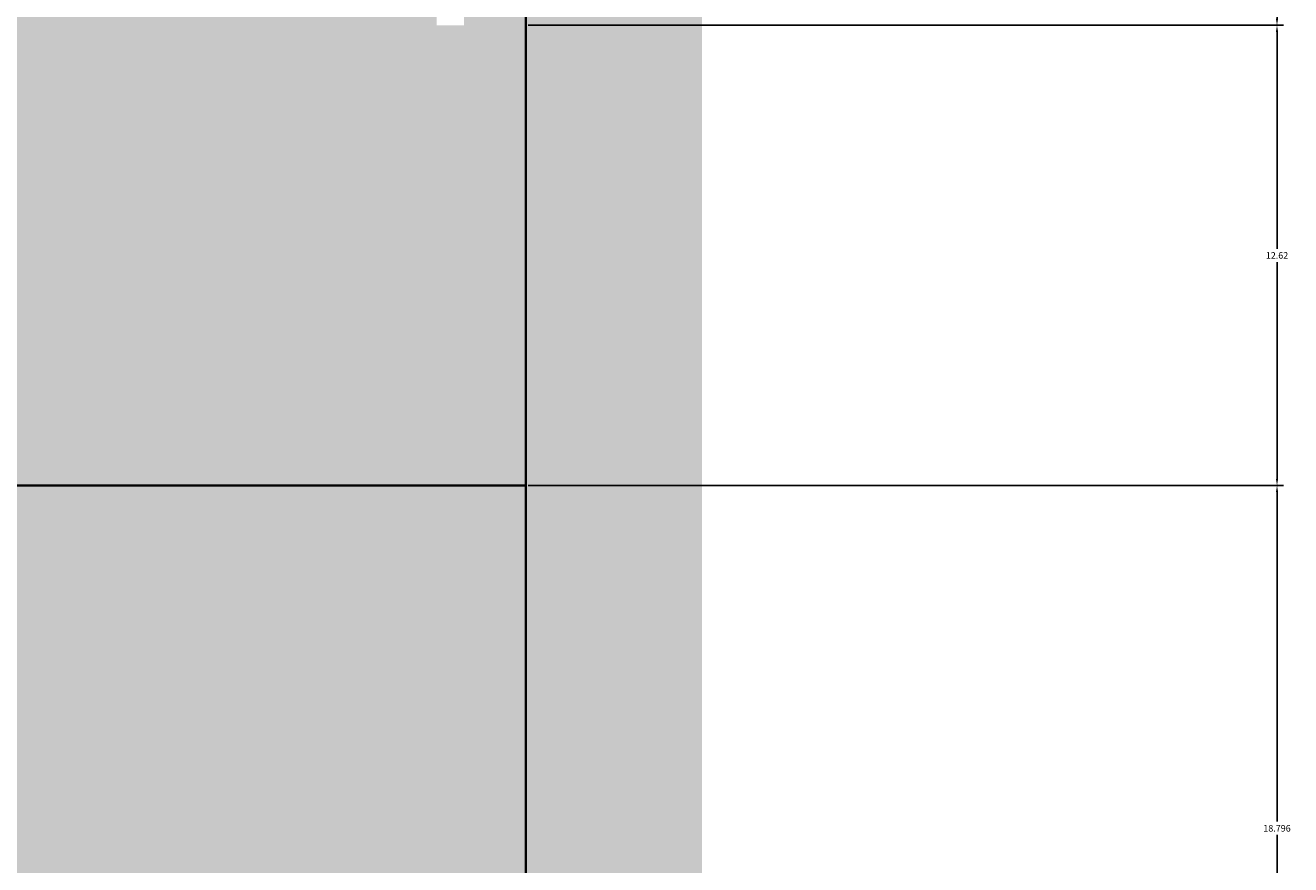
# Model space of a CAD drawing. Units: feet. Extents: x 2695 to 2912, y 795 to 1139.
# Tile 34 of 83: x 2877 to 2912, y 914 to 937. Entities that reach past the tile are written whole.
import ezdxf

# ---------------------------------------------------------------- set-up
doc = ezdxf.new("R2010")
doc.units = ezdxf.units.FT
for name, color, linetype, lineweight in [('A-ANNO-DIMS', 2, 'Continuous', 18), ('A-ELEV', 7, 'Continuous', 35), ('A-ELEV-PATT', 252, 'Continuous', 13)]:
    doc.layers.add(name, color=color, linetype=linetype, lineweight=lineweight)
doc.styles.get("Standard").update_dxf_attribs({"font": 'arial.ttf'})
doc.dimstyles.get("Standard").update_dxf_attribs({"dimtxt": 0.18, "dimasz": 0.18, "dimexe": 0.18, "dimexo": 0.0625, "dimgap": 0.09, "dimtad": 0, "dimtih": 1, "dimtoh": 1, "dimdec": 1, "dimzin": 0, "dimdsep": 46, "dimlunit": 3, "dimtxsty": 'Standard', "dimcen": 0.09, "dimadec": 0, "dimazin": 0, "dimtfac": 1, "dimtdec": 1, "dimtofl": 0, "dimtmove": 0, "dimatfit": 3, "dimfxl": 1, "dimtolj": 1, "dimtzin": 0, "dimarcsym": 0})

# ---------------------------------------------------------------- blocks, each defined once
blk = doc.blocks.new('*D15')
at = {"layer": 'A-ANNO-DIMS', "color": 0, "lineweight": -2, "transparency": 16777216}
for p, q in [((2890.699, 924.311), (2911.424, 924.311)), ((2911.244, 924.131), (2911.244, 915.094)), ((2911.244, 905.694), (2911.244, 914.731)), ((2838.439, 905.514), (2911.424, 905.514))]:
    blk.add_line(p, q, dxfattribs=at)
at = {"layer": 'A-ANNO-DIMS', "color": 0, "transparency": 16777216}
for points in [[(2911.214, 924.131), (2911.274, 924.131), (2911.244, 924.311)], [(2911.214, 905.694), (2911.274, 905.694), (2911.244, 905.514)]]:
    blk.add_solid(points, dxfattribs=at)
at = {"layer": 'Defpoints', "color": 0, "transparency": 16777216}
for p in [(2890.636, 924.311), (2911.244, 924.311), (2838.377, 905.514)]:
    blk.add_point(p, dxfattribs=at)
at = {"layer": 'A-ANNO-DIMS', "color": 0, "transparency": 16777216, "insert": (2911.244, 914.912), "char_height": 0.18, "attachment_point": 5}
blk.add_mtext('\\A1;18.796', dxfattribs=at)
blk = doc.blocks.new('*D16')
at = {"layer": 'A-ANNO-DIMS', "color": 0, "lineweight": -2, "transparency": 16777216}
for p, q in [((2890.699, 936.931), (2911.424, 936.931)), ((2911.244, 936.751), (2911.244, 930.802)), ((2911.244, 924.491), (2911.244, 930.439)), ((2890.699, 924.311), (2911.424, 924.311))]:
    blk.add_line(p, q, dxfattribs=at)
at = {"layer": 'A-ANNO-DIMS', "color": 0, "transparency": 16777216}
for points in [[(2911.214, 936.751), (2911.274, 936.751), (2911.244, 936.931)], [(2911.214, 924.491), (2911.274, 924.491), (2911.244, 924.311)]]:
    blk.add_solid(points, dxfattribs=at)
at = {"layer": 'Defpoints', "color": 0, "transparency": 16777216}
for p in [(2890.636, 936.931), (2911.244, 936.931), (2890.636, 924.311)]:
    blk.add_point(p, dxfattribs=at)
at = {"layer": 'A-ANNO-DIMS', "color": 0, "transparency": 16777216, "insert": (2911.244, 930.621), "char_height": 0.18, "attachment_point": 5}
blk.add_mtext('\\A1;12.62', dxfattribs=at)
blk = doc.blocks.new('*D17')
at = {"layer": 'A-ANNO-DIMS', "color": 0, "lineweight": -2, "transparency": 16777216}
for p, q in [((2843.637, 1020.824), (2911.424, 1020.824)), ((2911.244, 1020.644), (2911.244, 979.059)), ((2911.244, 937.111), (2911.244, 978.695)), ((2890.699, 936.931), (2911.424, 936.931))]:
    blk.add_line(p, q, dxfattribs=at)
at = {"layer": 'A-ANNO-DIMS', "color": 0, "transparency": 16777216}
for points in [[(2911.214, 1020.644), (2911.274, 1020.644), (2911.244, 1020.824)], [(2911.214, 937.111), (2911.274, 937.111), (2911.244, 936.931)]]:
    blk.add_solid(points, dxfattribs=at)
at = {"layer": 'Defpoints', "color": 0, "transparency": 16777216}
for p in [(2843.575, 1020.824), (2911.244, 1020.824), (2890.636, 936.931)]:
    blk.add_point(p, dxfattribs=at)
at = {"layer": 'A-ANNO-DIMS', "color": 0, "transparency": 16777216, "insert": (2911.244, 978.877), "char_height": 0.18, "attachment_point": 5}
blk.add_mtext('\\A1;83.9', dxfattribs=at)
blk = doc.blocks.new('*D53')
at = {"layer": 'A-ANNO-DIMS', "color": 0, "lineweight": -2, "transparency": 16777216}
for p, q in [((2890.699, 940.657), (2911.424, 940.657)), ((2911.244, 940.477), (2911.244, 938.976)), ((2911.244, 937.111), (2911.244, 938.612)), ((2890.699, 936.931), (2911.424, 936.931))]:
    blk.add_line(p, q, dxfattribs=at)
at = {"layer": 'A-ANNO-DIMS', "color": 0, "transparency": 16777216}
for points in [[(2911.214, 940.477), (2911.274, 940.477), (2911.244, 940.657)], [(2911.214, 937.111), (2911.274, 937.111), (2911.244, 936.931)]]:
    blk.add_solid(points, dxfattribs=at)
at = {"layer": 'Defpoints', "color": 0, "transparency": 16777216}
for p in [(2890.636, 940.657), (2911.244, 940.657), (2890.636, 936.931)]:
    blk.add_point(p, dxfattribs=at)
at = {"layer": 'A-ANNO-DIMS', "color": 0, "transparency": 16777216, "insert": (2911.244, 938.794), "char_height": 0.18, "attachment_point": 5}
blk.add_mtext('\\A1;3.726', dxfattribs=at)

msp = doc.modelspace()

# ---------------------------------------------------------------- hatches: boundary and pattern name
at = {"layer": 'A-ELEV-PATT'}
h = msp.add_hatch(color=256, dxfattribs=at)
h.set_gradient(color1=(255, 255, 255), tint=1)
h.paths.add_polyline_path([(2770.6361, 1122.9306), (2710.6361, 1122.9306), (2710.6361, 1118.4096), (2770.6361, 1118.4096)])
h.paths.add_polyline_path([(2890.6361, 1107.8588), (2770.6361, 1107.8588), (2770.6361, 1103.3378), (2890.6361, 1103.3378)])
h.paths.add_polyline_path([(2890.6361, 1062.9306), (2710.6361, 1062.9306), (2710.6361, 1056.9306), (2710.6361, 936.9306), (2710.6361, 924.3105), (2716.5358, 924.3105), (2890.6361, 924.3105), (2890.6361, 936.9306), (2715.8852, 936.9306), (2715.8852, 1050.3105), (2890.6361, 1050.3105)])
h.paths.add_polyline_path([(2716.5358, 924.3105), (2710.6361, 924.3105), (2710.6361, 810.9306), (2716.5358, 810.9306)])
h = msp.add_hatch(color=256, dxfattribs=at)
h.set_gradient(color1=(147, 149, 152), color2=(147, 149, 152), tint=1)
h.paths.add_polyline_path([(2770.6361, 1118.4096), (2710.6361, 1118.4096), (2710.6361, 1062.9306), (2770.6361, 1062.9306)])
h.paths.add_polyline_path([(2890.6361, 1103.3378), (2770.6361, 1103.3378), (2770.6361, 1062.9306), (2890.6361, 1062.9306)])
h.paths.add_polyline_path([(2730.7081, 1048.1052), (2755.1125, 1048.1052), (2755.1125, 936.9306), (2770.6361, 936.9306), (2770.6361, 1050.3105), (2715.8852, 1050.3105), (2715.8852, 936.9306), (2730.7081, 936.9306)])
h.paths.add_polyline_path([(2890.6361, 1050.3105), (2770.6361, 1050.3105), (2770.6361, 971.9673), (2778.0341, 971.9673), (2778.0341, 1020.8235), (2843.575, 1020.8235), (2843.575, 971.9673), (2890.6361, 971.9673)])
h.paths.add_polyline_path([(2888.1882, 970.7156), (2843.575, 970.7156), (2843.575, 964.8267), (2888.1882, 964.8267)])
h.paths.add_polyline_path([(2888.1882, 964.1328), (2843.575, 964.1328), (2843.575, 956.614), (2888.1882, 956.614)])
h.paths.add_polyline_path([(2888.1882, 955.9202), (2843.575, 955.9202), (2843.575, 949.2892), (2888.1882, 949.2892)])
h.paths.add_polyline_path([(2888.1882, 948.5954), (2843.575, 948.5954), (2843.575, 941.3507), (2888.1882, 941.3507)])
h.paths.add_polyline_path([(2888.1882, 940.6569), (2843.575, 940.6569), (2843.575, 936.9306), (2888.1882, 936.9306)])
h.paths.add_polyline_path([(2890.6361, 970.7156), (2888.9368, 970.7156), (2888.9368, 964.8267), (2890.6361, 964.8267)])
h.paths.add_polyline_path([(2890.6361, 964.1328), (2888.9368, 964.1328), (2888.9368, 956.614), (2890.6361, 956.614)])
h.paths.add_polyline_path([(2890.6361, 955.9202), (2888.9368, 955.9202), (2888.9368, 949.2892), (2890.6361, 949.2892)])
h.paths.add_polyline_path([(2890.6361, 940.6569), (2888.9368, 940.6569), (2888.9368, 936.9306), (2890.6361, 936.9306)])
h.paths.add_polyline_path([(2890.6361, 948.5954), (2888.9368, 948.5954), (2888.9368, 941.3507), (2890.6361, 941.3507)])
h.paths.add_polyline_path([(2772.5216, 970.7156), (2770.6361, 970.7156), (2770.6361, 964.8267), (2772.5216, 964.8267)])
h.paths.add_polyline_path([(2772.5216, 964.1328), (2770.6361, 964.1328), (2770.6361, 956.614), (2772.5216, 956.614)])
h.paths.add_polyline_path([(2772.5216, 955.9202), (2770.6361, 955.9202), (2770.6361, 949.2892), (2772.5216, 949.2892)])
h.paths.add_polyline_path([(2772.5216, 948.5954), (2770.6361, 948.5954), (2770.6361, 941.3507), (2772.5216, 941.3507)])
h.paths.add_polyline_path([(2772.5216, 940.6569), (2770.6361, 940.6569), (2770.6361, 936.9306), (2772.5216, 936.9306)])
h.paths.add_polyline_path([(2778.0341, 940.6569), (2773.2702, 940.6569), (2773.2702, 936.9306), (2778.0341, 936.9306)])
h.paths.add_polyline_path([(2778.0341, 970.7156), (2773.2702, 970.7156), (2773.2702, 964.8267), (2778.0341, 964.8267)])
h.paths.add_polyline_path([(2778.0341, 964.1328), (2773.2702, 964.1328), (2773.2702, 956.614), (2778.0341, 956.614)])
h.paths.add_polyline_path([(2778.0341, 955.9202), (2773.2702, 955.9202), (2773.2702, 949.2892), (2778.0341, 949.2892)])
h.paths.add_polyline_path([(2778.0341, 948.5954), (2773.2702, 948.5954), (2773.2702, 941.3507), (2778.0341, 941.3507)])
h.paths.add_polyline_path([(2810.0407, 940.6569), (2780.0341, 940.6569), (2780.0341, 936.9306), (2810.0407, 936.9306)])
h.paths.add_polyline_path([(2890.6361, 924.3105), (2770.6361, 924.3105), (2770.6361, 810.9306), (2773.5029, 810.9306), (2773.5029, 905.5143), (2805.9398, 905.5143), (2838.3767, 905.5143), (2838.3767, 810.9306), (2890.6361, 810.9306)])
h = msp.add_hatch(color=256, dxfattribs=at)
h.set_gradient(color1=(255, 255, 255), tint=1)
h.paths.add_polyline_path([(2895.4694, 1107.8588), (2890.6361, 1107.8588), (2890.6361, 810.9306), (2895.4694, 810.9306)])

# ---------------------------------------------------------------- linework, layer by layer
at = {"layer": 'A-ELEV'}
for p, q in [((2890.6361, 810.9306), (2890.6361, 1107.8588)), ((2890.6361, 1062.9306), (2890.6361, 810.9306))]:
    msp.add_line(p, q, dxfattribs=at)
msp.add_lwpolyline([(2890.6361, 936.9306), (2890.6361, 924.3105), (2710.6361, 924.3105), (2710.6361, 936.9306)], dxfattribs=at)

# ---------------------------------------------------------------- dimensions: what is measured, and where the dimension line sits
at = {"layer": 'A-ANNO-DIMS'}
for base, p1, p2, override, picture, middle in [((2911.2444, 1020.8235), (2890.6361, 936.9306), (2843.575, 1020.8235), {"dimdec": 1, "dimlfac": 1, "dimrnd": 0, "dimzin": 0, "dimdsep": 46, "dimlunit": 2}, '*D17', (2911.2444, 978.877)), ((2911.2444, 940.6569), (2890.6361, 936.9306), (2890.6361, 940.6569), {"dimdec": 3, "dimlfac": 1, "dimrnd": 0, "dimzin": 0, "dimdsep": 46, "dimlunit": 2}, '*D53', (2911.2444, 938.7937)), ((2911.2444, 936.9306), (2890.6361, 924.3105), (2890.6361, 936.9306), {"dimdec": 2, "dimlfac": 1, "dimrnd": 0, "dimzin": 0, "dimdsep": 46, "dimlunit": 2}, '*D16', (2911.2444, 930.6206)), ((2911.2444, 924.3105), (2838.3767, 905.5143), (2890.6361, 924.3105), {"dimdec": 3, "dimlfac": 1, "dimrnd": 0, "dimzin": 0, "dimdsep": 46, "dimlunit": 2}, '*D15', (2911.2444, 914.9124))]:
    dim = msp.add_linear_dim(base=base, p1=p1, p2=p2, angle=90, dimstyle='Standard', override=override, dxfattribs=at)
    dim.commit()
    dim.dimension.update_dxf_attribs({"geometry": picture, "text_midpoint": middle})

doc.saveas('drawing.dxf')
